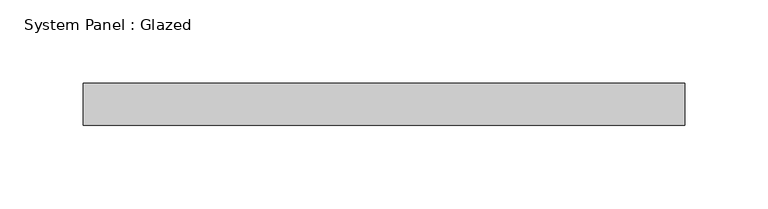
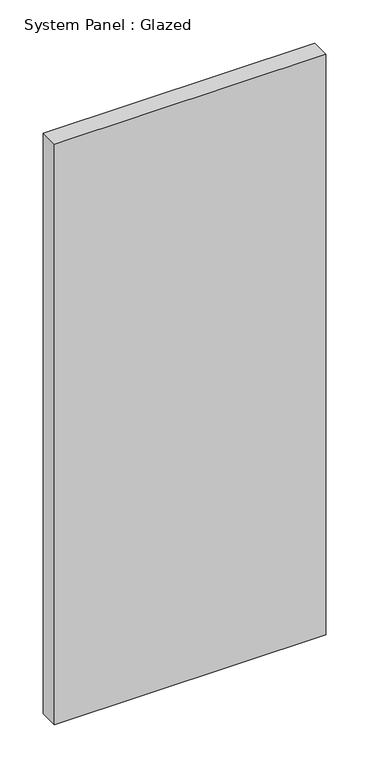
"""IFC4 building model written with IfcOpenShell, lengths in millimetres: plate geometry, System Panel : Glazed."""

from ifc_helpers import new_model, si_unit, origin, origin_with_axes, place, context, project, spatial, polyline, outline, extrude, source, transform, mapped, element, save


def system_panel_glazed_cc98a0ec(model_context):
    return source(origin(), model_context, "Body", "SweptSolid", [
        extrude(outline(polyline([(180.975, 19.05), (-180.975, 19.05), (-180.975, 44.45), (180.975, 44.45), (180.975, 19.05)])), origin_with_axes(), (0.0, 0.0, 1.0), 819.15),
    ])


if __name__ == "__main__":
    model = new_model("IFC4")
    model_context = context("Model", 3, world=origin())
    ifc_project = project(units=[si_unit("LENGTHUNIT", "METRE", prefix="MILLI")], contexts=[model_context])
    site = spatial("IfcSite", under=ifc_project)
    building = spatial("IfcBuilding", under=site)
    placement = place(None, origin())
    system_panel_glazed_shape = system_panel_glazed_cc98a0ec(model_context)
    element("IfcPlate", 1, ObjectType="System Panel : Glazed", at=placement, inside=building, context=model_context, shape_type="MappedRepresentation", body=[
        mapped(system_panel_glazed_shape, transform((0.0, 0.0, 0.0), x_axis=(1.0, 0.0, 0.0), y_axis=(0.0, 1.0, 0.0), z_axis=(0.0, 0.0, 1.0))),
    ])
    save(model, "model.ifc")

# Revit data of these elements
# Type "System Panel : Glazed"
#   Construction Type Id = "GSP4R"
#   Analytic Construction = "1/8 in Pilkington single glazing"
#   Visual Light Transmittance = 0.9
#   Solar Heat Gain Coefficient = 0.86
#   Heat Transfer Coefficient (U) = 1.18115 BTU/(h·ft²·°F)
#   Define Thermal Properties by = 1
# Element 1 (IfcPlate, "System Panel : Glazed")
#   Materials on its faces: "Glass"
# Materials
#   "Glass": class "Glass", colour RGB 0 128 192, transparency 0.75, Description = "Soda Lime Glass", Cost = 0
